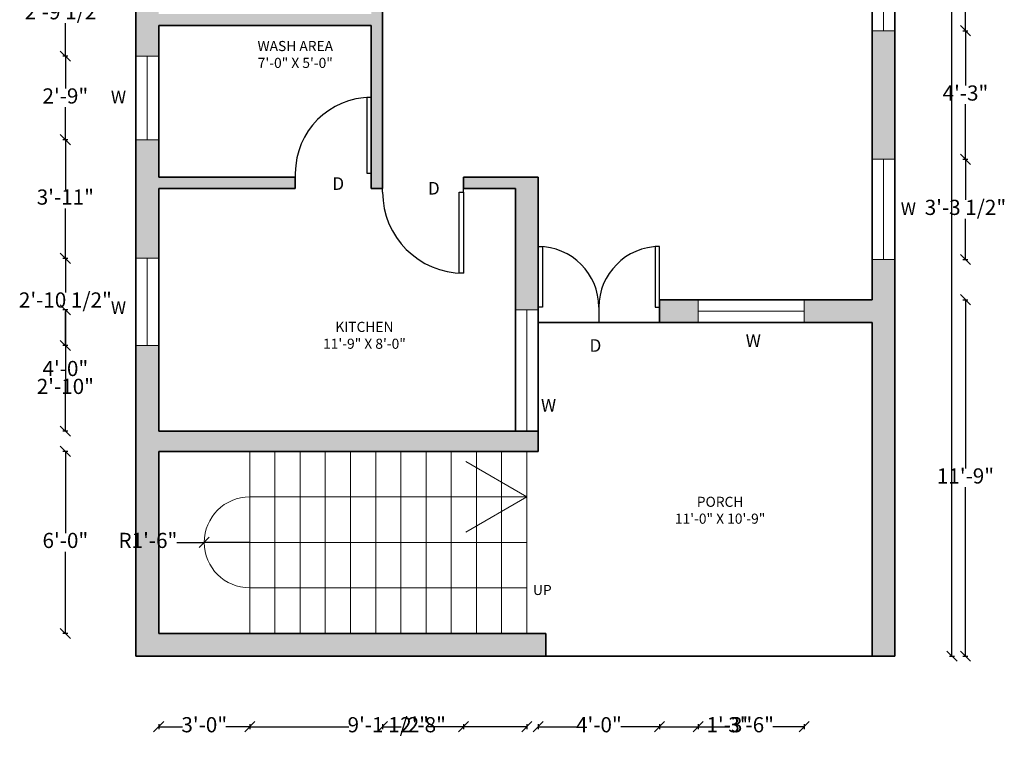
# Model space of a CAD drawing. Units: inches. Extents: x 2633 to 3023, y 679 to 1292.
# Tile 1 of 2: x 2633 to 3023, y 679 to 967. Entities that reach past the tile are written whole.
import ezdxf

# ---------------------------------------------------------------- set-up
doc = ezdxf.new("R2010")
doc.units = ezdxf.units.IN
for name, color, linetype, lineweight in [('A-ANNO-DIMS', 2, 'Continuous', 18), ('A-ANNO-TEXT', 7, 'Continuous', 18), ('A-AREA-IDEN', 7, 'Continuous', 18), ('A-DOOR', 4, 'Continuous', 25), ('A-FLOR-STRS', 7, 'Continuous', 18), ('A-GLAZ', 1, 'Continuous', 18), ('A-WALL', 7, 'Continuous', 35), ('A-WALL-PATT', 5, 'Continuous', 13)]:
    doc.layers.add(name, color=color, linetype=linetype, lineweight=lineweight)
doc.styles.get("Standard").update_dxf_attribs({"font": 'arial.ttf'})
doc.dimstyles.new('ISO-25', dxfattribs={"dimtxt": 6, "dimasz": 4, "dimexe": 1, "dimexo": 1, "dimtad": 0, "dimtih": 1, "dimtoh": 1, "dimlunit": 3, "dimtxsty": 'Standard', "dimblk": 'OBLIQUE', "dimcen": 2.5, "dimadec": 0, "dimazin": 0, "dimtfac": 1, "dimtmove": 0, "dimatfit": 3, "dimfxl": 1, "dimfxlon": 1, "dimarcsym": 0})

# ---------------------------------------------------------------- blocks, each defined once
blk = doc.blocks.new('*U5')
for p, q in [((-32, 0), (-32, 6)), ((0, 0), (0, 6))]:
    blk.add_line(p, q)
blk.add_lwpolyline([(0, 0), (0, -32), (-1.75, -32), (-1.75, 0)], close=True)
blk.add_arc((0, 0), 32, 180, 270)
blk = doc.blocks.new('*U7')
for p, q in [((-30, 0), (-30, -6)), ((0, 0), (0, -6))]:
    blk.add_line(p, q)
blk.add_lwpolyline([(0, 0), (0, 30), (-1.75, 30), (-1.75, 0)], close=True)
blk.add_arc((0, 0), 30, 90, 180)
blk = doc.blocks.new('*U6')
for p, q in [((0, 0), (0, -6)), ((24, 0), (24, -6))]:
    blk.add_line(p, q)
blk.add_lwpolyline([(0, 0), (0, 24), (1.75, 24), (1.75, 0)], close=True)
blk.add_arc((0, 0), 24, 0, 90)
blk = doc.blocks.new('*U4')
for p, q in [((-24, 0), (-24, -6)), ((0, 0), (0, -6))]:
    blk.add_line(p, q)
blk.add_lwpolyline([(0, 0), (0, 24), (-1.75, 24), (-1.75, 0)], close=True)
blk.add_arc((0, 0), 24, 90, 180)
blk = doc.blocks.new('_Oblique')
at = {"color": 0, "linetype": 'ByBlock', "lineweight": -2}
blk.add_line((-0.5, -0.5), (0.5, 0.5), dxfattribs=at)
blk = doc.blocks.new('*D12')
at = {"layer": 'A-ANNO-DIMS', "color": 0, "lineweight": -2, "transparency": 16777216}
for p, q in [((3000.92, 1255.4), (3002.92, 1255.4)), ((3001.92, 1255.4), (3001.92, 989.07)), ((3001.92, 715.4), (3001.92, 981.72)), ((3000.92, 715.4), (3002.92, 715.4))]:
    blk.add_line(p, q, dxfattribs=at)
at = {"layer": 'Defpoints', "color": 0, "transparency": 16777216}
for p in [(2979.35, 1255.4), (2979.35, 715.4), (3001.92, 715.4)]:
    blk.add_point(p, dxfattribs=at)
at = {"layer": 'A-ANNO-DIMS', "color": 0, "lineweight": -2, "transparency": 16777216, "xscale": 4, "yscale": 4, "zscale": 4}
for p, rotation in [((3001.92, 1255.4), 90), ((3001.92, 715.4), 270)]:
    blk.add_blockref('_Oblique', p, dxfattribs=dict(at, rotation=rotation))
at = {"layer": 'A-ANNO-DIMS', "color": 0, "transparency": 16777216, "insert": (3001.92, 985.4), "char_height": 6, "attachment_point": 5}
blk.add_mtext("45'", dxfattribs=at)
blk = doc.blocks.new('*D18')
at = {"layer": 'A-ANNO-DIMS', "color": 0, "lineweight": -2, "transparency": 16777216}
for p, q in [((2652.45, 796.4), (2650.45, 796.4)), ((2651.45, 796.4), (2651.45, 764.08)), ((2651.45, 724.4), (2651.45, 756.71)), ((2652.45, 724.4), (2650.45, 724.4))]:
    blk.add_line(p, q, dxfattribs=at)
at = {"layer": 'Defpoints', "color": 0, "transparency": 16777216}
for p in [(2651.45, 796.4), (2688.35, 796.4), (2688.35, 724.4)]:
    blk.add_point(p, dxfattribs=at)
at = {"layer": 'A-ANNO-DIMS', "color": 0, "lineweight": -2, "transparency": 16777216, "xscale": 4, "yscale": 4, "zscale": 4}
for p, rotation in [((2651.45, 796.4), 90), ((2651.45, 724.4), 270)]:
    blk.add_blockref('_Oblique', p, dxfattribs=dict(at, rotation=rotation))
at = {"layer": 'A-ANNO-DIMS', "color": 0, "transparency": 16777216, "insert": (2651.45, 760.4), "char_height": 6, "attachment_point": 5}
blk.add_mtext('6\'-0"', dxfattribs=at)
blk = doc.blocks.new('*D19')
at = {"layer": 'A-ANNO-DIMS', "color": 0, "lineweight": -2, "transparency": 16777216}
for p, q in [((2688.35, 688.5), (2688.35, 686.5)), ((2688.35, 687.5), (2697.75, 687.5)), ((2724.35, 687.5), (2714.94, 687.5)), ((2724.35, 688.5), (2724.35, 686.5))]:
    blk.add_line(p, q, dxfattribs=at)
at = {"layer": 'Defpoints', "color": 0, "transparency": 16777216}
for p in [(2688.35, 724.4), (2724.35, 724.4), (2724.35, 687.5)]:
    blk.add_point(p, dxfattribs=at)
at = {"layer": 'A-ANNO-DIMS', "color": 0, "lineweight": -2, "transparency": 16777216, "xscale": 4, "yscale": 4, "zscale": 4, "rotation": 180}
blk.add_blockref('_Oblique', (2688.35, 687.5), dxfattribs=at)
at = {"layer": 'A-ANNO-DIMS', "color": 0, "lineweight": -2, "transparency": 16777216, "xscale": 4, "yscale": 4, "zscale": 4}
blk.add_blockref('_Oblique', (2724.35, 687.5), dxfattribs=at)
at = {"layer": 'A-ANNO-DIMS', "color": 0, "transparency": 16777216, "insert": (2706.35, 687.5), "char_height": 6, "attachment_point": 5}
blk.add_mtext('3\'-0"', dxfattribs=at)
blk = doc.blocks.new('*D20')
at = {"layer": 'A-ANNO-DIMS', "color": 0, "lineweight": -2, "transparency": 16777216}
for p, q in [((2724.35, 1282.3), (2724.35, 1284.3)), ((2724.35, 1283.3), (2734.3, 1283.3)), ((2734.3, 1282.3), (2734.3, 1284.3)), ((2734.3, 1283.3), (2738.3, 1283.3))]:
    blk.add_line(p, q, dxfattribs=at)
at = {"layer": 'Defpoints', "color": 0, "transparency": 16777216}
for p in [(2734.3, 1283.3), (2724.35, 724.4), (2734.3, 724.4)]:
    blk.add_point(p, dxfattribs=at)
at = {"layer": 'A-ANNO-DIMS', "color": 0, "lineweight": -2, "transparency": 16777216, "xscale": 4, "yscale": 4, "zscale": 4, "rotation": 180}
blk.add_blockref('_Oblique', (2724.35, 1283.3), dxfattribs=at)
at = {"layer": 'A-ANNO-DIMS', "color": 0, "lineweight": -2, "transparency": 16777216, "xscale": 4, "yscale": 4, "zscale": 4}
blk.add_blockref('_Oblique', (2734.3, 1283.3), dxfattribs=at)
at = {"layer": 'A-ANNO-DIMS', "color": 0, "transparency": 16777216, "insert": (2749.23, 1283.3), "char_height": 6, "attachment_point": 5}
blk.add_mtext('0\'-10"', dxfattribs=at)
blk = doc.blocks.new('*D21')
at = {"layer": 'A-ANNO-DIMS', "color": 0, "lineweight": -2, "transparency": 16777216}
for p, q in [((2724.35, 688.5), (2724.35, 686.5)), ((2724.35, 687.5), (2763.51, 687.5)), ((2833.85, 687.5), (2794.69, 687.5)), ((2833.85, 688.5), (2833.85, 686.5))]:
    blk.add_line(p, q, dxfattribs=at)
at = {"layer": 'Defpoints', "color": 0, "transparency": 16777216}
for p in [(2724.35, 724.4), (2833.85, 724.4), (2833.85, 687.5)]:
    blk.add_point(p, dxfattribs=at)
at = {"layer": 'A-ANNO-DIMS', "color": 0, "lineweight": -2, "transparency": 16777216, "xscale": 4, "yscale": 4, "zscale": 4, "rotation": 180}
blk.add_blockref('_Oblique', (2724.35, 687.5), dxfattribs=at)
at = {"layer": 'A-ANNO-DIMS', "color": 0, "lineweight": -2, "transparency": 16777216, "xscale": 4, "yscale": 4, "zscale": 4}
blk.add_blockref('_Oblique', (2833.85, 687.5), dxfattribs=at)
at = {"layer": 'A-ANNO-DIMS', "color": 0, "transparency": 16777216, "insert": (2779.1, 687.5), "char_height": 6, "attachment_point": 5}
blk.add_mtext('9\'-1 1/2"', dxfattribs=at)
blk = doc.blocks.new('*D22')
at = {"layer": 'A-ANNO-DIMS', "color": 0, "lineweight": -2, "transparency": 16777216}
for p, q in [((2838.35, 688.5), (2838.35, 686.5)), ((2838.35, 687.5), (2853.63, 687.5)), ((2886.35, 687.5), (2871.07, 687.5)), ((2886.35, 688.5), (2886.35, 686.5))]:
    blk.add_line(p, q, dxfattribs=at)
at = {"layer": 'Defpoints', "color": 0, "transparency": 16777216}
for p in [(2838.35, 847.4), (2886.35, 847.4), (2886.35, 687.5)]:
    blk.add_point(p, dxfattribs=at)
at = {"layer": 'A-ANNO-DIMS', "color": 0, "lineweight": -2, "transparency": 16777216, "xscale": 4, "yscale": 4, "zscale": 4, "rotation": 180}
blk.add_blockref('_Oblique', (2838.35, 687.5), dxfattribs=at)
at = {"layer": 'A-ANNO-DIMS', "color": 0, "lineweight": -2, "transparency": 16777216, "xscale": 4, "yscale": 4, "zscale": 4}
blk.add_blockref('_Oblique', (2886.35, 687.5), dxfattribs=at)
at = {"layer": 'A-ANNO-DIMS', "color": 0, "transparency": 16777216, "insert": (2862.35, 687.5), "char_height": 6, "attachment_point": 5}
blk.add_mtext('4\'-0"', dxfattribs=at)
blk = doc.blocks.new('*D24')
at = {"layer": 'A-ANNO-DIMS', "color": 0, "lineweight": -2, "transparency": 16777216}
for p, q in [((2776.85, 688.5), (2776.85, 686.5)), ((2776.85, 687.5), (2784.2, 687.5)), ((2808.85, 687.5), (2801.5, 687.5)), ((2808.85, 688.5), (2808.85, 686.5))]:
    blk.add_line(p, q, dxfattribs=at)
at = {"layer": 'Defpoints', "color": 0, "transparency": 16777216}
for p in [(2776.85, 900.4), (2808.85, 900.4), (2808.85, 687.5)]:
    blk.add_point(p, dxfattribs=at)
at = {"layer": 'A-ANNO-DIMS', "color": 0, "lineweight": -2, "transparency": 16777216, "xscale": 4, "yscale": 4, "zscale": 4, "rotation": 180}
blk.add_blockref('_Oblique', (2776.85, 687.5), dxfattribs=at)
at = {"layer": 'A-ANNO-DIMS', "color": 0, "lineweight": -2, "transparency": 16777216, "xscale": 4, "yscale": 4, "zscale": 4}
blk.add_blockref('_Oblique', (2808.85, 687.5), dxfattribs=at)
at = {"layer": 'A-ANNO-DIMS', "color": 0, "transparency": 16777216, "insert": (2792.85, 687.5), "char_height": 6, "attachment_point": 5}
blk.add_mtext('2\'-8"', dxfattribs=at)
blk = doc.blocks.new('*D25')
at = {"layer": 'A-ANNO-DIMS', "color": 0, "lineweight": -2, "transparency": 16777216}
for p, q in [((2742.35, 1282.3), (2742.35, 1284.3)), ((2742.35, 1283.3), (2748.7, 1283.3)), ((2772.35, 1283.3), (2766, 1283.3)), ((2772.35, 1282.3), (2772.35, 1284.3))]:
    blk.add_line(p, q, dxfattribs=at)
at = {"layer": 'Defpoints', "color": 0, "transparency": 16777216}
for p in [(2772.35, 1283.3), (2742.35, 904.9), (2772.35, 904.65)]:
    blk.add_point(p, dxfattribs=at)
at = {"layer": 'A-ANNO-DIMS', "color": 0, "lineweight": -2, "transparency": 16777216, "xscale": 4, "yscale": 4, "zscale": 4, "rotation": 180}
blk.add_blockref('_Oblique', (2742.35, 1283.3), dxfattribs=at)
at = {"layer": 'A-ANNO-DIMS', "color": 0, "lineweight": -2, "transparency": 16777216, "xscale": 4, "yscale": 4, "zscale": 4}
blk.add_blockref('_Oblique', (2772.35, 1283.3), dxfattribs=at)
at = {"layer": 'A-ANNO-DIMS', "color": 0, "transparency": 16777216, "insert": (2757.35, 1283.3), "char_height": 6, "attachment_point": 5}
blk.add_mtext('2\'-6"', dxfattribs=at)
blk = doc.blocks.new('*D29')
at = {"layer": 'A-ANNO-DIMS', "color": 0, "lineweight": -2, "transparency": 16777216}
for p, q in [((2652.45, 838.24), (2650.45, 838.24)), ((2651.45, 838.24), (2651.45, 825.01)), ((2651.45, 804.4), (2651.45, 817.63)), ((2652.45, 804.4), (2650.45, 804.4))]:
    blk.add_line(p, q, dxfattribs=at)
at = {"layer": 'Defpoints', "color": 0, "transparency": 16777216}
for p in [(2651.45, 838.24), (2688.35, 838.24), (2688.35, 804.4)]:
    blk.add_point(p, dxfattribs=at)
at = {"layer": 'A-ANNO-DIMS', "color": 0, "lineweight": -2, "transparency": 16777216, "xscale": 4, "yscale": 4, "zscale": 4}
for p, rotation in [((2651.45, 838.24), 90), ((2651.45, 804.4), 270)]:
    blk.add_blockref('_Oblique', p, dxfattribs=dict(at, rotation=rotation))
at = {"layer": 'A-ANNO-DIMS', "color": 0, "transparency": 16777216, "insert": (2651.45, 821.32), "char_height": 6, "attachment_point": 5}
blk.add_mtext('2\'-10"', dxfattribs=at)
blk = doc.blocks.new('*D30')
at = {"layer": 'A-ANNO-DIMS', "color": 0, "lineweight": -2, "transparency": 16777216}
for p, q in [((2652.45, 872.75), (2650.45, 872.75)), ((2651.45, 872.75), (2651.45, 859.22)), ((2651.45, 838.24), (2651.45, 851.77)), ((2652.45, 838.24), (2650.45, 838.24))]:
    blk.add_line(p, q, dxfattribs=at)
at = {"layer": 'Defpoints', "color": 0, "transparency": 16777216}
for p in [(2651.45, 872.75), (2679.35, 872.75), (2679.35, 838.24)]:
    blk.add_point(p, dxfattribs=at)
at = {"layer": 'A-ANNO-DIMS', "color": 0, "lineweight": -2, "transparency": 16777216, "xscale": 4, "yscale": 4, "zscale": 4}
for p, rotation in [((2651.45, 872.75), 90), ((2651.45, 838.24), 270)]:
    blk.add_blockref('_Oblique', p, dxfattribs=dict(at, rotation=rotation))
at = {"layer": 'A-ANNO-DIMS', "color": 0, "transparency": 16777216, "insert": (2651.45, 855.5), "char_height": 6, "attachment_point": 5}
blk.add_mtext('2\'-10 1/2"', dxfattribs=at)
blk = doc.blocks.new('*D31')
at = {"layer": 'A-ANNO-DIMS', "color": 0, "lineweight": -2, "transparency": 16777216}
for p, q in [((2652.45, 919.67), (2650.45, 919.67)), ((2651.45, 919.67), (2651.45, 899.9)), ((2651.45, 872.75), (2651.45, 892.52)), ((2652.45, 872.75), (2650.45, 872.75))]:
    blk.add_line(p, q, dxfattribs=at)
at = {"layer": 'Defpoints', "color": 0, "transparency": 16777216}
for p in [(2651.45, 919.67), (2679.35, 919.67), (2679.35, 872.75)]:
    blk.add_point(p, dxfattribs=at)
at = {"layer": 'A-ANNO-DIMS', "color": 0, "lineweight": -2, "transparency": 16777216, "xscale": 4, "yscale": 4, "zscale": 4}
for p, rotation in [((2651.45, 919.67), 90), ((2651.45, 872.75), 270)]:
    blk.add_blockref('_Oblique', p, dxfattribs=dict(at, rotation=rotation))
at = {"layer": 'A-ANNO-DIMS', "color": 0, "transparency": 16777216, "insert": (2651.45, 896.21), "char_height": 6, "attachment_point": 5}
blk.add_mtext('3\'-11"', dxfattribs=at)
blk = doc.blocks.new('*D32')
at = {"layer": 'A-ANNO-DIMS', "color": 0, "lineweight": -2, "transparency": 16777216}
for p, q in [((2652.45, 952.74), (2650.45, 952.74)), ((2651.45, 952.74), (2651.45, 939.89)), ((2651.45, 919.67), (2651.45, 932.51)), ((2652.45, 919.67), (2650.45, 919.67))]:
    blk.add_line(p, q, dxfattribs=at)
at = {"layer": 'Defpoints', "color": 0, "transparency": 16777216}
for p in [(2651.45, 952.74), (2679.35, 952.74), (2679.35, 919.67)]:
    blk.add_point(p, dxfattribs=at)
at = {"layer": 'A-ANNO-DIMS', "color": 0, "lineweight": -2, "transparency": 16777216, "xscale": 4, "yscale": 4, "zscale": 4}
for p, rotation in [((2651.45, 952.74), 90), ((2651.45, 919.67), 270)]:
    blk.add_blockref('_Oblique', p, dxfattribs=dict(at, rotation=rotation))
at = {"layer": 'A-ANNO-DIMS', "color": 0, "transparency": 16777216, "insert": (2651.45, 936.2), "char_height": 6, "attachment_point": 5}
blk.add_mtext('2\'-9"', dxfattribs=at)
blk = doc.blocks.new('*D33')
at = {"layer": 'A-ANNO-DIMS', "color": 0, "lineweight": -2, "transparency": 16777216}
for p, q in [((2652.45, 986.26), (2650.45, 986.26)), ((2651.45, 986.26), (2651.45, 973.23)), ((2651.45, 952.74), (2651.45, 965.77)), ((2652.45, 952.74), (2650.45, 952.74))]:
    blk.add_line(p, q, dxfattribs=at)
at = {"layer": 'Defpoints', "color": 0, "transparency": 16777216}
for p in [(2651.45, 986.26), (2679.35, 986.26), (2679.35, 952.74)]:
    blk.add_point(p, dxfattribs=at)
at = {"layer": 'A-ANNO-DIMS', "color": 0, "lineweight": -2, "transparency": 16777216, "xscale": 4, "yscale": 4, "zscale": 4}
for p, rotation in [((2651.45, 986.26), 90), ((2651.45, 952.74), 270)]:
    blk.add_blockref('_Oblique', p, dxfattribs=dict(at, rotation=rotation))
at = {"layer": 'A-ANNO-DIMS', "color": 0, "transparency": 16777216, "insert": (2651.45, 969.5), "char_height": 6, "attachment_point": 5}
blk.add_mtext('2\'-9 1/2"', dxfattribs=at)
blk = doc.blocks.new('*D39')
at = {"layer": 'A-ANNO-DIMS', "color": 0, "lineweight": -2, "transparency": 16777216}
for p, q in [((3006.25, 856.4), (3008.25, 856.4)), ((3007.25, 856.4), (3007.25, 789.58)), ((3007.25, 715.4), (3007.25, 782.21)), ((3006.25, 715.4), (3008.25, 715.4))]:
    blk.add_line(p, q, dxfattribs=at)
at = {"layer": 'Defpoints', "color": 0, "transparency": 16777216}
for p in [(2970.35, 856.4), (3007.25, 856.4), (2970.35, 715.4)]:
    blk.add_point(p, dxfattribs=at)
at = {"layer": 'A-ANNO-DIMS', "color": 0, "lineweight": -2, "transparency": 16777216, "xscale": 4, "yscale": 4, "zscale": 4}
for p, rotation in [((3007.25, 856.4), 90), ((3007.25, 715.4), 270)]:
    blk.add_blockref('_Oblique', p, dxfattribs=dict(at, rotation=rotation))
at = {"layer": 'A-ANNO-DIMS', "color": 0, "transparency": 16777216, "insert": (3007.25, 785.9), "char_height": 6, "attachment_point": 5}
blk.add_mtext('11\'-9"', dxfattribs=at)
blk = doc.blocks.new('*D40')
at = {"layer": 'A-ANNO-DIMS', "color": 0, "lineweight": -2, "transparency": 16777216}
for p, q in [((3006.25, 911.93), (3008.25, 911.93)), ((3007.25, 911.93), (3007.25, 895.85)), ((3007.25, 872.32), (3007.25, 888.4)), ((3006.25, 872.32), (3008.25, 872.32))]:
    blk.add_line(p, q, dxfattribs=at)
at = {"layer": 'Defpoints', "color": 0, "transparency": 16777216}
for p in [(2979.35, 911.93), (3007.25, 911.93), (2979.35, 872.32)]:
    blk.add_point(p, dxfattribs=at)
at = {"layer": 'A-ANNO-DIMS', "color": 0, "lineweight": -2, "transparency": 16777216, "xscale": 4, "yscale": 4, "zscale": 4}
for p, rotation in [((3007.25, 911.93), 90), ((3007.25, 872.32), 270)]:
    blk.add_blockref('_Oblique', p, dxfattribs=dict(at, rotation=rotation))
at = {"layer": 'A-ANNO-DIMS', "color": 0, "transparency": 16777216, "insert": (3007.25, 892.13), "char_height": 6, "attachment_point": 5}
blk.add_mtext('3\'-3 1/2"', dxfattribs=at)
blk = doc.blocks.new('*D41')
at = {"layer": 'A-ANNO-DIMS', "color": 0, "lineweight": -2, "transparency": 16777216}
for p, q in [((3006.25, 962.79), (3008.25, 962.79)), ((3007.25, 962.79), (3007.25, 941.05)), ((3007.25, 911.93), (3007.25, 933.67)), ((3006.25, 911.93), (3008.25, 911.93))]:
    blk.add_line(p, q, dxfattribs=at)
at = {"layer": 'Defpoints', "color": 0, "transparency": 16777216}
for p in [(2979.35, 962.79), (3007.25, 962.79), (2979.35, 911.93)]:
    blk.add_point(p, dxfattribs=at)
at = {"layer": 'A-ANNO-DIMS', "color": 0, "lineweight": -2, "transparency": 16777216, "xscale": 4, "yscale": 4, "zscale": 4}
for p, rotation in [((3007.25, 962.79), 90), ((3007.25, 911.93), 270)]:
    blk.add_blockref('_Oblique', p, dxfattribs=dict(at, rotation=rotation))
at = {"layer": 'A-ANNO-DIMS', "color": 0, "transparency": 16777216, "insert": (3007.25, 937.36), "char_height": 6, "attachment_point": 5}
blk.add_mtext('4\'-3"', dxfattribs=at)
blk = doc.blocks.new('*D42')
at = {"layer": 'A-ANNO-DIMS', "color": 0, "lineweight": -2, "transparency": 16777216}
for p, q in [((3006.25, 1008.83), (3008.25, 1008.83)), ((3007.25, 1008.83), (3007.25, 989.5)), ((3007.25, 962.79), (3007.25, 982.12)), ((3006.25, 962.79), (3008.25, 962.79))]:
    blk.add_line(p, q, dxfattribs=at)
at = {"layer": 'Defpoints', "color": 0, "transparency": 16777216}
for p in [(2979.35, 1008.83), (3007.25, 1008.83), (2979.35, 962.79)]:
    blk.add_point(p, dxfattribs=at)
at = {"layer": 'A-ANNO-DIMS', "color": 0, "lineweight": -2, "transparency": 16777216, "xscale": 4, "yscale": 4, "zscale": 4}
for p, rotation in [((3007.25, 1008.83), 90), ((3007.25, 962.79), 270)]:
    blk.add_blockref('_Oblique', p, dxfattribs=dict(at, rotation=rotation))
at = {"layer": 'A-ANNO-DIMS', "color": 0, "transparency": 16777216, "insert": (3007.25, 985.81), "char_height": 6, "attachment_point": 5}
blk.add_mtext('3\'-10"', dxfattribs=at)
blk = doc.blocks.new('*D48')
at = {"layer": 'A-ANNO-DIMS', "color": 0, "lineweight": -2, "transparency": 16777216}
for p, q in [((2901.59, 688.5), (2901.59, 686.5)), ((2901.59, 687.5), (2913.93, 687.5)), ((2943.46, 687.5), (2931.12, 687.5)), ((2943.46, 688.5), (2943.46, 686.5))]:
    blk.add_line(p, q, dxfattribs=at)
at = {"layer": 'Defpoints', "color": 0, "transparency": 16777216}
for p in [(2901.59, 847.4), (2943.46, 847.4), (2943.46, 687.5)]:
    blk.add_point(p, dxfattribs=at)
at = {"layer": 'A-ANNO-DIMS', "color": 0, "lineweight": -2, "transparency": 16777216, "xscale": 4, "yscale": 4, "zscale": 4, "rotation": 180}
blk.add_blockref('_Oblique', (2901.59, 687.5), dxfattribs=at)
at = {"layer": 'A-ANNO-DIMS', "color": 0, "lineweight": -2, "transparency": 16777216, "xscale": 4, "yscale": 4, "zscale": 4}
blk.add_blockref('_Oblique', (2943.46, 687.5), dxfattribs=at)
at = {"layer": 'A-ANNO-DIMS', "color": 0, "transparency": 16777216, "insert": (2922.52, 687.5), "char_height": 6, "attachment_point": 5}
blk.add_mtext('3\'-6"', dxfattribs=at)
blk = doc.blocks.new('*D49')
at = {"layer": 'A-ANNO-DIMS', "color": 0, "lineweight": -2, "transparency": 16777216}
for p, q in [((2886.35, 688.5), (2886.35, 686.5)), ((2886.35, 687.5), (2901.59, 687.5)), ((2901.59, 688.5), (2901.59, 686.5)), ((2901.59, 687.5), (2905.59, 687.5))]:
    blk.add_line(p, q, dxfattribs=at)
at = {"layer": 'Defpoints', "color": 0, "transparency": 16777216}
for p in [(2886.35, 847.4), (2901.59, 847.4), (2901.59, 687.5)]:
    blk.add_point(p, dxfattribs=at)
at = {"layer": 'A-ANNO-DIMS', "color": 0, "lineweight": -2, "transparency": 16777216, "xscale": 4, "yscale": 4, "zscale": 4, "rotation": 180}
blk.add_blockref('_Oblique', (2886.35, 687.5), dxfattribs=at)
at = {"layer": 'A-ANNO-DIMS', "color": 0, "lineweight": -2, "transparency": 16777216, "xscale": 4, "yscale": 4, "zscale": 4}
blk.add_blockref('_Oblique', (2901.59, 687.5), dxfattribs=at)
at = {"layer": 'A-ANNO-DIMS', "color": 0, "transparency": 16777216, "insert": (2913.91, 687.5), "char_height": 6, "attachment_point": 5}
blk.add_mtext('1\'-3"', dxfattribs=at)
blk = doc.blocks.new('*D50')
at = {"layer": 'A-ANNO-DIMS', "color": 0, "lineweight": -2, "transparency": 16777216}
for p, q in [((2652.45, 852.4), (2650.45, 852.4)), ((2651.45, 852.4), (2651.45, 832.08)), ((2651.45, 804.4), (2651.45, 824.71)), ((2652.45, 804.4), (2650.45, 804.4))]:
    blk.add_line(p, q, dxfattribs=at)
at = {"layer": 'Defpoints', "color": 0, "transparency": 16777216}
for p in [(2651.45, 852.4), (2829.35, 852.4), (2829.35, 804.4)]:
    blk.add_point(p, dxfattribs=at)
at = {"layer": 'A-ANNO-DIMS', "color": 0, "lineweight": -2, "transparency": 16777216, "xscale": 4, "yscale": 4, "zscale": 4}
for p, rotation in [((2651.45, 852.4), 90), ((2651.45, 804.4), 270)]:
    blk.add_blockref('_Oblique', p, dxfattribs=dict(at, rotation=rotation))
at = {"layer": 'A-ANNO-DIMS', "color": 0, "transparency": 16777216, "insert": (2651.45, 828.4), "char_height": 6, "attachment_point": 5}
blk.add_mtext('4\'-0"', dxfattribs=at)
blk = doc.blocks.new('*D51')
at = {"layer": 'A-ANNO-DIMS', "color": 0, "lineweight": -2, "transparency": 16777216}
for p in [(2695.55, 760.4), (2724.35, 760.4)]:
    blk.add_line(p, (2706.35, 760.4), dxfattribs=at)
at = {"layer": 'Defpoints', "color": 0, "transparency": 16777216}
for p in [(2706.35, 760.4), (2724.35, 760.4)]:
    blk.add_point(p, dxfattribs=at)
at = {"layer": 'A-ANNO-DIMS', "color": 0, "lineweight": -2, "transparency": 16777216, "xscale": 4, "yscale": 4, "zscale": 4, "rotation": 359.9995670985548}
blk.add_blockref('_Oblique', (2706.35, 760.4), dxfattribs=at)
at = {"layer": 'A-ANNO-DIMS', "color": 0, "transparency": 16777216, "insert": (2684.08, 760.4), "char_height": 6, "attachment_point": 5}
blk.add_mtext('R1\'-6"', dxfattribs=at)

msp = doc.modelspace()

# ---------------------------------------------------------------- hatches: boundary and pattern name
at = {"layer": 'A-WALL-PATT'}
h = msp.add_hatch(color=256, dxfattribs=at)
h.dxf.hatch_style = 1
h.paths.add_polyline_path([(2777.347, 1246.396), (2777.347, 1216.396), (2781.847, 1216.396), (2781.847, 1246.396), (2824.847, 1246.396), (2824.847, 1029.396), (2833.847, 1029.396), (2833.847, 1246.396), (2876.847, 1246.396), (2876.847, 1216.396), (2881.347, 1216.396), (2881.347, 1246.396), (2970.347, 1246.396), (2970.347, 1236.412), (2979.347, 1236.412), (2979.347, 1255.396), (2679.347, 1255.396), (2679.347, 1227.707), (2688.347, 1227.707), (2688.347, 1246.396)])
h.paths.add_polyline_path([(2688.347, 1033.896), (2688.347, 1084.661), (2679.347, 1084.661), (2679.347, 1013.042), (2688.347, 1013.042), (2688.347, 1029.396), (2776.847, 1029.396), (2788.847, 1029.396), (2788.847, 1033.896)])
h.paths.add_polyline_path([(2679.347, 952.735), (2688.347, 952.735), (2688.347, 964.896), (2772.347, 964.896), (2772.347, 900.396), (2776.847, 900.396), (2776.847, 964.896), (2776.847, 999.396), (2772.347, 999.396), (2772.347, 969.396), (2688.347, 969.396), (2688.347, 986.261), (2679.347, 986.261)])
h.paths.add_polyline_path([(2688.347, 1181.896), (2781.847, 1181.896), (2781.847, 1186.396), (2688.347, 1186.396), (2688.347, 1198.143), (2679.347, 1198.143), (2679.347, 1144.586), (2688.347, 1144.586)], flags=17)
h.paths.add_polyline_path([(2688.347, 900.396), (2742.347, 900.396), (2742.347, 904.896), (2688.347, 904.896), (2688.347, 919.665), (2679.347, 919.665), (2679.347, 872.753), (2688.347, 872.753)])
h.paths.add_polyline_path([(2679.347, 715.396), (2841.347, 715.396), (2841.347, 724.396), (2688.347, 724.396), (2688.347, 796.396), (2838.347, 796.396), (2838.347, 804.396), (2829.347, 804.396), (2688.347, 804.396), (2688.347, 838.241), (2679.347, 838.241)])
h.paths.add_polyline_path([(2838.347, 904.896), (2808.847, 904.896), (2808.847, 900.396), (2829.347, 900.396), (2829.347, 852.396), (2838.347, 852.396)])
h.paths.add_polyline_path([(2970.347, 856.396), (2943.46, 856.396), (2943.46, 847.396), (2970.347, 847.396), (2970.347, 715.396), (2979.347, 715.396), (2979.347, 872.317), (2970.347, 872.317)])
h.paths.add_polyline_path([(2979.347, 962.792), (2970.347, 962.792), (2970.347, 911.933), (2979.347, 911.933)])
h.paths.add_polyline_path([(2979.347, 1081.378), (2970.347, 1081.378), (2970.347, 1033.896), (2869.847, 1033.896), (2869.847, 1029.396), (2970.347, 1029.396), (2970.347, 1008.832), (2979.347, 1008.832)])
h.paths.add_polyline_path([(2979.347, 1205.007), (2970.347, 1205.007), (2970.347, 1186.396), (2876.847, 1186.396), (2876.847, 1181.896), (2970.347, 1181.896), (2970.347, 1154.2), (2979.347, 1154.2)], flags=17)
h.paths.add_polyline_path([(2901.589, 847.396), (2901.589, 856.396), (2886.347, 856.396), (2886.347, 847.396)])

# ---------------------------------------------------------------- linework, layer by layer
at = {"layer": 'A-FLOR-STRS'}
for p, q in [((2724.347, 796.396), (2724.347, 724.396)), ((2734.302, 796.396), (2734.302, 724.396)), ((2744.256, 796.396), (2744.256, 724.396)), ((2754.211, 796.396), (2754.211, 724.396)), ((2764.165, 796.396), (2764.165, 724.396)), ((2774.12, 796.396), (2774.12, 724.396)), ((2784.074, 796.396), (2784.074, 724.396)), ((2794.029, 796.396), (2794.029, 724.396)), ((2803.983, 796.396), (2803.983, 724.396)), ((2813.938, 796.396), (2813.938, 724.396)), ((2823.893, 796.396), (2823.893, 724.396)), ((2833.847, 796.396), (2833.847, 724.396)), ((2833.847, 778.396), (2809.715, 792.328)), ((2724.347, 778.396), (2833.847, 778.396)), ((2833.847, 778.396), (2809.715, 764.463)), ((2833.847, 760.396), (2724.347, 760.396)), ((2833.847, 742.396), (2724.347, 742.396))]:
    msp.add_line(p, q, dxfattribs=at)
msp.add_arc((2724.347, 760.396), 18, 90, 270, dxfattribs=at)
at = {"layer": 'A-GLAZ'}
for p, q in [((2974.847, 1008.832), (2974.847, 962.792)), ((2970.347, 962.792), (2979.347, 962.792)), ((2688.347, 952.735), (2679.347, 952.735)), ((2683.847, 919.665), (2683.847, 952.735)), ((2688.347, 919.665), (2679.347, 919.665)), ((2970.347, 911.933), (2979.347, 911.933)), ((2974.847, 911.933), (2974.847, 872.317)), ((2688.347, 872.753), (2679.347, 872.753)), ((2683.847, 838.241), (2683.847, 872.753)), ((2970.347, 872.317), (2979.347, 872.317)), ((2901.589, 856.396), (2901.589, 847.396)), ((2943.46, 856.396), (2943.46, 847.396)), ((2829.347, 852.396), (2838.347, 852.396)), ((2833.847, 852.396), (2833.847, 804.396)), ((2901.589, 851.896), (2943.46, 851.896)), ((2688.347, 838.241), (2679.347, 838.241)), ((2829.347, 804.396), (2838.347, 804.396))]:
    msp.add_line(p, q, dxfattribs=at)
at = {"layer": 'A-WALL'}
for p, q in [((2679.347, 1255.396), (2679.347, 715.396)), ((2979.347, 715.396), (2979.347, 1255.396)), ((2776.847, 1029.396), (2776.847, 964.896)), ((2970.347, 856.396), (2970.347, 1029.396)), ((2772.347, 964.896), (2688.347, 964.896)), ((2688.347, 964.896), (2688.347, 904.896)), ((2772.347, 964.896), (2772.347, 900.396)), ((2776.847, 964.896), (2776.847, 900.396)), ((2742.347, 904.896), (2688.347, 904.896)), ((2742.347, 900.396), (2742.347, 904.896)), ((2838.347, 904.896), (2808.847, 904.896)), ((2808.847, 904.896), (2808.847, 900.396)), ((2838.347, 904.896), (2838.347, 847.396)), ((2688.347, 900.396), (2688.347, 804.396)), ((2742.347, 900.396), (2688.347, 900.396)), ((2776.847, 900.396), (2772.347, 900.396)), ((2829.347, 900.396), (2808.847, 900.396)), ((2829.347, 900.396), (2829.347, 804.396)), ((2886.347, 856.396), (2970.347, 856.396)), ((2886.347, 847.396), (2886.347, 856.396)), ((2838.347, 847.396), (2970.347, 847.396)), ((2838.347, 847.396), (2838.347, 796.396)), ((2970.347, 715.396), (2970.347, 847.396)), ((2838.347, 804.396), (2688.347, 804.396)), ((2838.347, 796.396), (2688.347, 796.396)), ((2688.347, 796.396), (2688.347, 724.396)), ((2688.347, 724.396), (2841.347, 724.396)), ((2841.347, 715.396), (2841.347, 724.396)), ((2679.347, 715.396), (2979.347, 715.396))]:
    msp.add_line(p, q, dxfattribs=at)

# ---------------------------------------------------------------- block references
at = {"layer": 'A-DOOR'}
for name, p in [('*U7', (2772.347, 906.396)), ('*U5', (2808.847, 898.896)), ('*U6', (2838.347, 853.396)), ('*U4', (2886.347, 853.396))]:
    msp.add_blockref(name, p, dxfattribs=at)

# ---------------------------------------------------------------- texts
at = {"layer": 'A-ANNO-TEXT', "attachment_point": 1}
for s, width, insert, char_height in [('\\pxqc;W', 6.8199, (2669.038, 939.037), 5), ('\\pxqc;D', 6.8199, (2755.893, 904.815), 5), ('\\pxqc;D', 6.8199, (2793.671, 902.957), 5), ('\\pxqc;W', 6.8199, (2981.274, 894.853), 5), ('\\pxqc;W', 6.8199, (2669.038, 855.774), 5), ('\\pxqc;D', 6.8199, (2857.572, 840.772), 5), ('\\pxqc;W', 6.8199, (2919.977, 842.687), 5), ('\\pxqc;W', 6.8199, (2839.042, 817.159), 5), ('UP', 7.19581, (2836.287, 743.582), 4)]:
    msp.add_mtext_dynamic_manual_height_columns(s, width=width, gutter_width=12.5, heights=[0], dxfattribs=dict(at, insert=insert, char_height=char_height))
at = {"layer": 'A-AREA-IDEN', "char_height": 4, "attachment_point": 1}
for s, width, insert in [('\\pxqc;WASH AREA\\P7\'-0" X 5\'-0"', 33.8072, (2725.432, 958.726)), ('\\pxqc;KITCHEN\\P11\'-9" X 8\'-0"', 33.8072, (2752.772, 847.637)), ('\\pxqc;PORCH\\P11\'-0" X 10\'-9"', 37.05921, (2891.736, 778.442))]:
    msp.add_mtext_dynamic_manual_height_columns(s, width=width, gutter_width=12.5, heights=[0], dxfattribs=dict(at, insert=insert))

# ---------------------------------------------------------------- dimensions: what is measured, and where the dimension line sits
at = {"layer": 'A-ANNO-DIMS'}
for base, p1, p2, picture, middle in [((2734.302, 1283.296), (2724.347, 724.396), (2734.302, 724.396), '*D20', (2749.232, 1283.296)), ((2772.347, 1283.296), (2742.347, 904.896), (2772.347, 904.646), '*D25', (2757.347, 1283.296)), ((2808.847, 687.496), (2776.847, 900.396), (2808.847, 900.396), '*D24', (2792.847, 687.496)), ((2886.347, 687.496), (2838.347, 847.396), (2886.347, 847.396), '*D22', (2862.347, 687.496)), ((2901.589, 687.496), (2886.347, 847.396), (2901.589, 847.396), '*D49', (2913.906, 687.496)), ((2943.46, 687.496), (2901.589, 847.396), (2943.46, 847.396), '*D48', (2922.524, 687.496)), ((2724.347, 687.496), (2688.347, 724.396), (2724.347, 724.396), '*D19', (2706.347, 687.496)), ((2833.847, 687.496), (2724.347, 724.396), (2833.847, 724.396), '*D21', (2779.097, 687.496))]:
    dim = msp.add_linear_dim(base=base, p1=p1, p2=p2, dimstyle='ISO-25', override={"dimdec": 1, "dimlfac": 1, "dimrnd": 0, "dimzin": 1, "dimdsep": 46, "dimlunit": 4, "dimfrac": 2}, dxfattribs=at)
    dim.commit()
    dim.dimension.update_dxf_attribs({"geometry": picture, "text_midpoint": middle})
for base, p1, p2, override, picture, middle in [((3001.916, 715.396), (2979.347, 1255.396), (2979.347, 715.396), {"dimclrd": 0, "dimclre": 0, "dimclrt": 0}, '*D12', (3001.916, 985.396)), ((3007.247, 1008.832), (2979.347, 962.792), (2979.347, 1008.832), {"dimdec": 1, "dimlfac": 1, "dimrnd": 0, "dimzin": 1, "dimdsep": 46, "dimlunit": 4, "dimfrac": 2}, '*D42', (3007.247, 985.812)), ((2651.447, 986.261), (2679.347, 952.735), (2679.347, 986.261), {"dimdec": 1, "dimlfac": 1, "dimrnd": 0, "dimzin": 1, "dimdsep": 46, "dimlunit": 4, "dimfrac": 2}, '*D33', (2651.447, 969.498)), ((3007.247, 962.792), (2979.347, 911.933), (2979.347, 962.792), {"dimdec": 1, "dimlfac": 1, "dimrnd": 0, "dimzin": 1, "dimdsep": 46, "dimlunit": 4, "dimfrac": 2}, '*D41', (3007.247, 937.363)), ((2651.447, 952.735), (2679.347, 919.665), (2679.347, 952.735), {"dimdec": 1, "dimlfac": 1, "dimrnd": 0, "dimzin": 1, "dimdsep": 46, "dimlunit": 4, "dimfrac": 2}, '*D32', (2651.447, 936.2)), ((2651.447, 919.665), (2679.347, 872.753), (2679.347, 919.665), {"dimdec": 1, "dimlfac": 1, "dimrnd": 0, "dimzin": 1, "dimdsep": 46, "dimlunit": 4, "dimfrac": 2}, '*D31', (2651.447, 896.209)), ((3007.247, 911.933), (2979.347, 872.317), (2979.347, 911.933), {"dimdec": 1, "dimlfac": 1, "dimrnd": 0, "dimzin": 1, "dimdsep": 46, "dimlunit": 4, "dimfrac": 2}, '*D40', (3007.247, 892.125)), ((2651.447, 872.753), (2679.347, 838.241), (2679.347, 872.753), {"dimdec": 1, "dimlfac": 1, "dimrnd": 0, "dimzin": 1, "dimdsep": 46, "dimlunit": 4, "dimfrac": 2}, '*D30', (2651.447, 855.497)), ((3007.247, 856.396), (2970.347, 715.396), (2970.347, 856.396), {"dimdec": 1, "dimlfac": 1, "dimrnd": 0, "dimzin": 1, "dimdsep": 46, "dimlunit": 4, "dimfrac": 2}, '*D39', (3007.247, 785.896)), ((2651.447, 852.396), (2829.347, 804.396), (2829.347, 852.396), {"dimdec": 1, "dimlfac": 1, "dimrnd": 0, "dimzin": 1, "dimdsep": 46, "dimlunit": 4, "dimfrac": 2}, '*D50', (2651.447, 828.396)), ((2651.447, 838.241), (2688.347, 804.396), (2688.347, 838.241), {"dimdec": 1, "dimlfac": 1, "dimrnd": 0, "dimzin": 1, "dimdsep": 46, "dimlunit": 4, "dimfrac": 2}, '*D29', (2651.447, 821.318)), ((2651.447, 796.396), (2688.347, 724.396), (2688.347, 796.396), {"dimdec": 1, "dimlfac": 1, "dimrnd": 0, "dimzin": 1, "dimdsep": 46, "dimlunit": 4, "dimfrac": 2}, '*D18', (2651.447, 760.396))]:
    dim = msp.add_linear_dim(base=base, p1=p1, p2=p2, angle=90, dimstyle='ISO-25', override=override, dxfattribs=at)
    dim.commit()
    dim.dimension.update_dxf_attribs({"geometry": picture, "text_midpoint": middle})
dim = msp.add_radius_dim(center=(2724.347, 760.396), mpoint=(2706.347, 760.396), dimstyle='ISO-25', override={"dimdec": 1, "dimlfac": 1, "dimrnd": 0, "dimzin": 1, "dimdsep": 46, "dimlunit": 4, "dimfrac": 2}, dxfattribs=at)
dim.commit()
dim.dimension.update_dxf_attribs({"geometry": '*D51', "text_midpoint": (2695.547, 760.396), "dimtype": 164})

doc.saveas('drawing.dxf')
